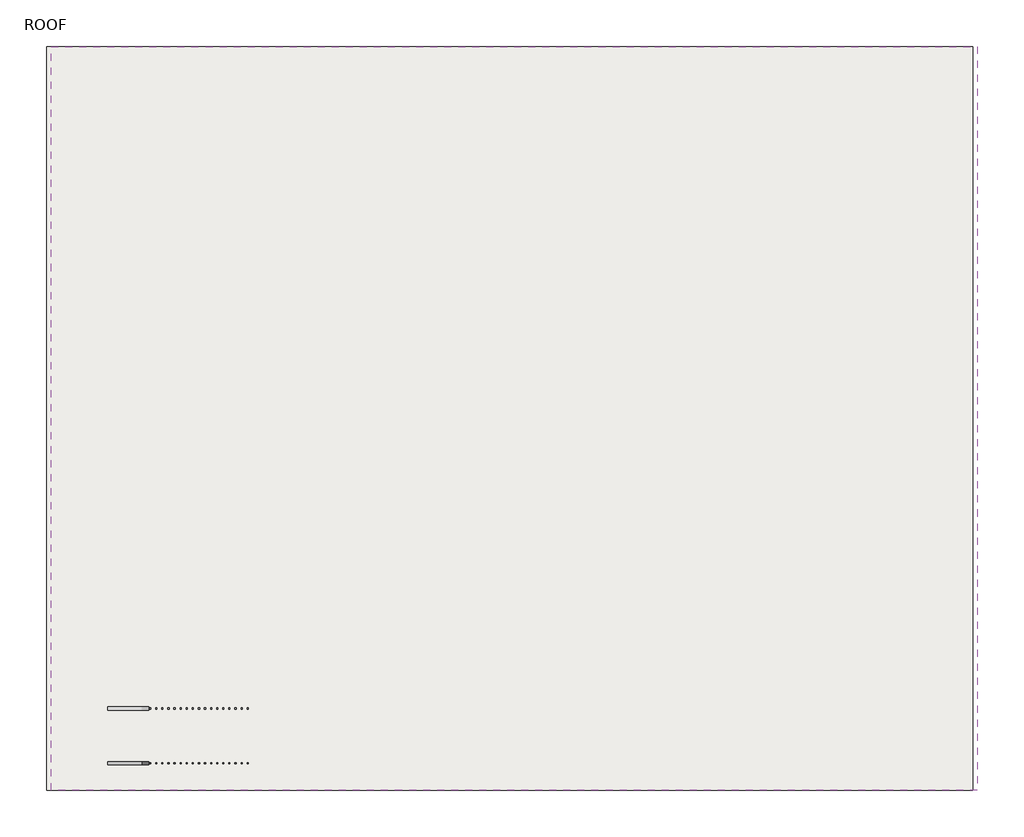
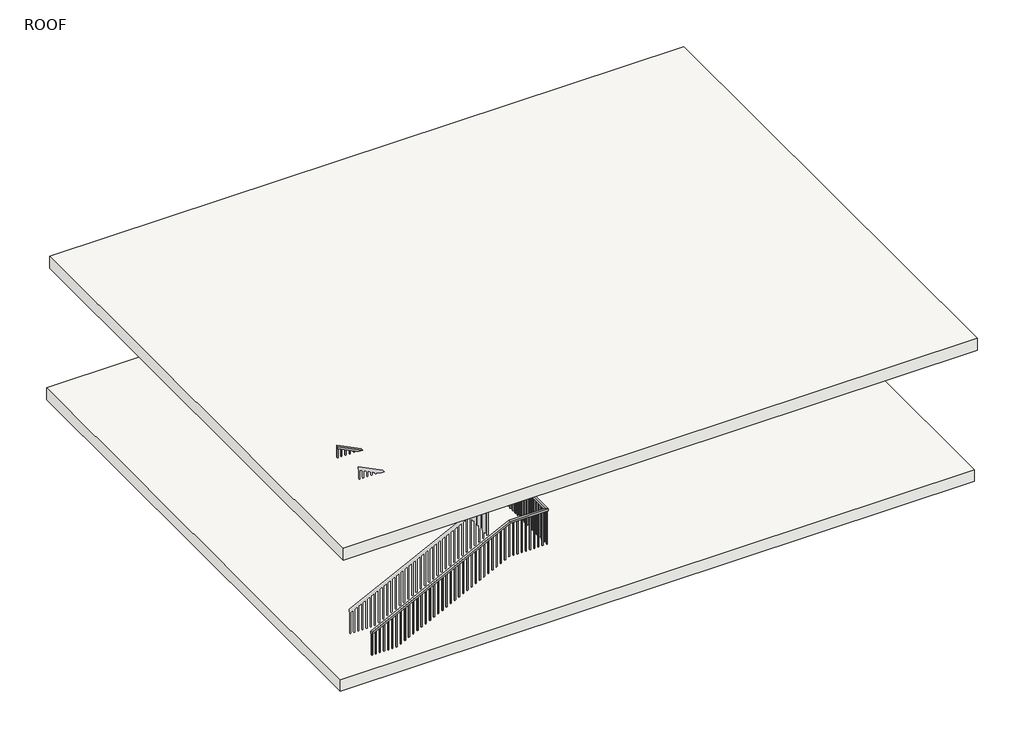
# One storey, part 1 of 2: 2 slabs, 1 railing.
"""IFC4 building model written with IfcOpenShell, lengths in millimetres."""

from ifc_helpers import new_model, si_unit, frame, origin, place, context, project, spatial, polyline, outline, extrude, faceted_brep, element, save

model = new_model("IFC4")

# Units and contexts
model_context = context("Model", 3, world=origin())
ifc_project = project(units=[si_unit("LENGTHUNIT", "METRE", prefix="MILLI")], contexts=[model_context])

# Site, building, storey
site = spatial("IfcSite", under=ifc_project)
building = spatial("IfcBuilding", under=site)
storey = spatial("IfcBuildingStorey", under=building, Name="ROOF", Elevation=12192.0)

# Railing
placement = place(None, origin())
element("IfcRailing", 1, ObjectType="Handrail - Rectangular", at=placement, inside=storey, context=model_context, shape_type="SolidModel", body=[
    faceted_brep([(-8362.2800418, -5370.1090076, 13106.4), (-8362.2800418, -5370.1090076, 13049.6038734), (-8362.2800418, -5420.9090076, 13049.6038734), (-8362.2800418, -5420.9090076, 13106.4), (-5009.4800418, -5370.1090076, 14782.8), (-4997.4877885, -5370.1090076, 14732.0), (-4997.4877885, -5420.9090076, 14732.0), (-5009.4800418, -5420.9090076, 14782.8), (-4120.4800418, -5370.1090076, 14782.8), (-4120.4800418, -5370.1090076, 14732.0), (-4069.6800418, -5420.9090076, 14732.0), (-4069.6800418, -5420.9090076, 14782.8), (-4120.4800418, -2917.1346494, 14782.8), (-4120.4800418, -2917.1346494, 14732.0), (-4069.6800418, -2866.3346494, 14732.0), (-4069.6800418, -2866.3346494, 14782.8), (-5009.4800418, -2917.1346494, 14782.8), (-5021.472295, -2917.1346494, 14732.0), (-5021.472295, -2866.3346494, 14732.0), (-5009.4800418, -2866.3346494, 14782.8), (-7752.6800418, -2917.1346494, 16154.4), (-7752.6800418, -2866.3346494, 16154.4), (-7752.6800418, -2866.3346494, 16097.6038734), (-7752.6800418, -2917.1346494, 16097.6038734)], [[[0, 1, 2, 3]], [[1, 0, 4, 5]], [[2, 1, 5, 6]], [[3, 2, 6, 7]], [[0, 3, 7, 4]], [[5, 4, 8, 9]], [[6, 5, 9, 10]], [[7, 6, 10, 11]], [[4, 7, 11, 8]], [[9, 8, 12, 13]], [[10, 9, 13, 14]], [[11, 10, 14, 15]], [[8, 11, 15, 12]], [[13, 12, 16, 17]], [[14, 13, 17, 18]], [[15, 14, 18, 19]], [[12, 15, 19, 16]], [[20, 21, 22, 23]], [[17, 16, 20, 23]], [[18, 17, 23, 22]], [[19, 18, 22, 21]], [[16, 19, 21, 20]]]),
    extrude(outline(polyline([(16051.5663734, -7660.6050418), (15193.9625, -7660.6050418), (15184.4375, -7641.5550418), (16042.0413734, -7641.5550418), (16051.5663734, -7660.6050418)])), frame((0.0, -2901.2596494, 0.0), z_axis=(0.0, 1.0, 0.0), x_axis=(0.0, 0.0, 1.0)), (0.0, 0.0, 1.0), 19.05),
    extrude(outline(polyline([(16000.7663734, -7559.0050418), (15143.1625, -7559.0050418), (15133.6375, -7539.9550418), (15991.2413734, -7539.9550418), (16000.7663734, -7559.0050418)])), frame((0.0, -2901.2596494, 0.0), z_axis=(0.0, 1.0, 0.0), x_axis=(0.0, 0.0, 1.0)), (0.0, 0.0, 1.0), 19.05),
    extrude(outline(polyline([(15949.9663734, -7457.4050418), (15092.3625, -7457.4050418), (15082.8375, -7438.3550418), (15940.4413734, -7438.3550418), (15949.9663734, -7457.4050418)])), frame((0.0, -2901.2596494, 0.0), z_axis=(0.0, 1.0, 0.0), x_axis=(0.0, 0.0, 1.0)), (0.0, 0.0, 1.0), 19.05),
    extrude(outline(polyline([(15899.1663734, -7355.8050418), (15041.5625, -7355.8050418), (15032.0375, -7336.7550418), (15889.6413734, -7336.7550418), (15899.1663734, -7355.8050418)])), frame((0.0, -2901.2596494, 0.0), z_axis=(0.0, 1.0, 0.0), x_axis=(0.0, 0.0, 1.0)), (0.0, 0.0, 1.0), 19.05),
    extrude(outline(polyline([(15848.3663734, -7254.2050418), (14990.7625, -7254.2050418), (14981.2375, -7235.1550418), (15838.8413734, -7235.1550418), (15848.3663734, -7254.2050418)])), frame((0.0, -2901.2596494, 0.0), z_axis=(0.0, 1.0, 0.0), x_axis=(0.0, 0.0, 1.0)), (0.0, 0.0, 1.0), 19.05),
    extrude(outline(polyline([(15797.5663734, -7152.6050418), (14939.9625, -7152.6050418), (14930.4375, -7133.5550418), (15788.0413734, -7133.5550418), (15797.5663734, -7152.6050418)])), frame((0.0, -2901.2596494, 0.0), z_axis=(0.0, 1.0, 0.0), x_axis=(0.0, 0.0, 1.0)), (0.0, 0.0, 1.0), 19.05),
    extrude(outline(polyline([(15746.7663734, -7051.0050418), (14889.1625, -7051.0050418), (14879.6375, -7031.9550418), (15737.2413734, -7031.9550418), (15746.7663734, -7051.0050418)])), frame((0.0, -2901.2596494, 0.0), z_axis=(0.0, 1.0, 0.0), x_axis=(0.0, 0.0, 1.0)), (0.0, 0.0, 1.0), 19.05),
    extrude(outline(polyline([(15695.9663734, -6949.4050418), (14838.3625, -6949.4050418), (14828.8375, -6930.3550418), (15686.4413734, -6930.3550418), (15695.9663734, -6949.4050418)])), frame((0.0, -2901.2596494, 0.0), z_axis=(0.0, 1.0, 0.0), x_axis=(0.0, 0.0, 1.0)), (0.0, 0.0, 1.0), 19.05),
    extrude(outline(polyline([(15645.1663734, -6847.8050418), (14787.5625, -6847.8050418), (14778.0375, -6828.7550418), (15635.6413734, -6828.7550418), (15645.1663734, -6847.8050418)])), frame((0.0, -2901.2596494, 0.0), z_axis=(0.0, 1.0, 0.0), x_axis=(0.0, 0.0, 1.0)), (0.0, 0.0, 1.0), 19.05),
    extrude(outline(polyline([(15594.3663734, -6746.2050418), (14736.7625, -6746.2050418), (14727.2375, -6727.1550418), (15584.8413734, -6727.1550418), (15594.3663734, -6746.2050418)])), frame((0.0, -2901.2596494, 0.0), z_axis=(0.0, 1.0, 0.0), x_axis=(0.0, 0.0, 1.0)), (0.0, 0.0, 1.0), 19.05),
    extrude(outline(polyline([(15543.5663734, -6644.6050418), (14685.9625, -6644.6050418), (14676.4375, -6625.5550418), (15534.0413734, -6625.5550418), (15543.5663734, -6644.6050418)])), frame((0.0, -2901.2596494, 0.0), z_axis=(0.0, 1.0, 0.0), x_axis=(0.0, 0.0, 1.0)), (0.0, 0.0, 1.0), 19.05),
    extrude(outline(polyline([(15492.7663734, -6543.0050418), (14635.1625, -6543.0050418), (14625.6375, -6523.9550418), (15483.2413734, -6523.9550418), (15492.7663734, -6543.0050418)])), frame((0.0, -2901.2596494, 0.0), z_axis=(0.0, 1.0, 0.0), x_axis=(0.0, 0.0, 1.0)), (0.0, 0.0, 1.0), 19.05),
    extrude(outline(polyline([(15441.9663734, -6441.4050418), (14584.3625, -6441.4050418), (14574.8375, -6422.3550418), (15432.4413734, -6422.3550418), (15441.9663734, -6441.4050418)])), frame((0.0, -2901.2596494, 0.0), z_axis=(0.0, 1.0, 0.0), x_axis=(0.0, 0.0, 1.0)), (0.0, 0.0, 1.0), 19.05),
    extrude(outline(polyline([(15391.1663734, -6339.8050418), (14533.5625, -6339.8050418), (14524.0375, -6320.7550418), (15381.6413734, -6320.7550418), (15391.1663734, -6339.8050418)])), frame((0.0, -2901.2596494, 0.0), z_axis=(0.0, 1.0, 0.0), x_axis=(0.0, 0.0, 1.0)), (0.0, 0.0, 1.0), 19.05),
    extrude(outline(polyline([(15340.3663734, -6238.2050418), (14482.7625, -6238.2050418), (14473.2375, -6219.1550418), (15330.8413734, -6219.1550418), (15340.3663734, -6238.2050418)])), frame((0.0, -2901.2596494, 0.0), z_axis=(0.0, 1.0, 0.0), x_axis=(0.0, 0.0, 1.0)), (0.0, 0.0, 1.0), 19.05),
    extrude(outline(polyline([(15289.5663734, -6136.6050418), (14431.9625, -6136.6050418), (14422.4375, -6117.5550418), (15280.0413734, -6117.5550418), (15289.5663734, -6136.6050418)])), frame((0.0, -2901.2596494, 0.0), z_axis=(0.0, 1.0, 0.0), x_axis=(0.0, 0.0, 1.0)), (0.0, 0.0, 1.0), 19.05),
    extrude(outline(polyline([(15238.7663734, -6035.0050418), (14381.1625, -6035.0050418), (14371.6375, -6015.9550418), (15229.2413734, -6015.9550418), (15238.7663734, -6035.0050418)])), frame((0.0, -2901.2596494, 0.0), z_axis=(0.0, 1.0, 0.0), x_axis=(0.0, 0.0, 1.0)), (0.0, 0.0, 1.0), 19.05),
    extrude(outline(polyline([(15187.9663734, -5933.4050418), (14330.3625, -5933.4050418), (14320.8375, -5914.3550418), (15178.4413734, -5914.3550418), (15187.9663734, -5933.4050418)])), frame((0.0, -2901.2596494, 0.0), z_axis=(0.0, 1.0, 0.0), x_axis=(0.0, 0.0, 1.0)), (0.0, 0.0, 1.0), 19.05),
    extrude(outline(polyline([(15137.1663734, -5831.8050418), (14279.5625, -5831.8050418), (14270.0375, -5812.7550418), (15127.6413734, -5812.7550418), (15137.1663734, -5831.8050418)])), frame((0.0, -2901.2596494, 0.0), z_axis=(0.0, 1.0, 0.0), x_axis=(0.0, 0.0, 1.0)), (0.0, 0.0, 1.0), 19.05),
    extrude(outline(polyline([(15086.3663734, -5730.2050418), (14228.7625, -5730.2050418), (14219.2375, -5711.1550418), (15076.8413734, -5711.1550418), (15086.3663734, -5730.2050418)])), frame((0.0, -2901.2596494, 0.0), z_axis=(0.0, 1.0, 0.0), x_axis=(0.0, 0.0, 1.0)), (0.0, 0.0, 1.0), 19.05),
    extrude(outline(polyline([(15035.5663734, -5628.6050418), (14177.9625, -5628.6050418), (14168.4375, -5609.5550418), (15026.0413734, -5609.5550418), (15035.5663734, -5628.6050418)])), frame((0.0, -2901.2596494, 0.0), z_axis=(0.0, 1.0, 0.0), x_axis=(0.0, 0.0, 1.0)), (0.0, 0.0, 1.0), 19.05),
    extrude(outline(polyline([(14984.7663734, -5527.0050418), (14127.1625, -5527.0050418), (14117.6375, -5507.9550418), (14975.2413734, -5507.9550418), (14984.7663734, -5527.0050418)])), frame((0.0, -2901.2596494, 0.0), z_axis=(0.0, 1.0, 0.0), x_axis=(0.0, 0.0, 1.0)), (0.0, 0.0, 1.0), 19.05),
    extrude(outline(polyline([(14933.9663734, -5425.4050418), (14076.3625, -5425.4050418), (14066.8375, -5406.3550418), (14924.4413734, -5406.3550418), (14933.9663734, -5425.4050418)])), frame((0.0, -2901.2596494, 0.0), z_axis=(0.0, 1.0, 0.0), x_axis=(0.0, 0.0, 1.0)), (0.0, 0.0, 1.0), 19.05),
    extrude(outline(polyline([(14883.1663734, -5323.8050418), (14025.5625, -5323.8050418), (14016.0375, -5304.7550418), (14873.6413734, -5304.7550418), (14883.1663734, -5323.8050418)])), frame((0.0, -2901.2596494, 0.0), z_axis=(0.0, 1.0, 0.0), x_axis=(0.0, 0.0, 1.0)), (0.0, 0.0, 1.0), 19.05),
    extrude(outline(polyline([(14832.3663734, -5222.2050418), (13974.7625, -5222.2050418), (13965.2375, -5203.1550418), (14822.8413734, -5203.1550418), (14832.3663734, -5222.2050418)])), frame((0.0, -2901.2596494, 0.0), z_axis=(0.0, 1.0, 0.0), x_axis=(0.0, 0.0, 1.0)), (0.0, 0.0, 1.0), 19.05),
    extrude(outline(polyline([(14781.5663734, -5120.6050418), (13923.9625, -5120.6050418), (13914.4375, -5101.5550418), (14772.0413734, -5101.5550418), (14781.5663734, -5120.6050418)])), frame((0.0, -2901.2596494, 0.0), z_axis=(0.0, 1.0, 0.0), x_axis=(0.0, 0.0, 1.0)), (0.0, 0.0, 1.0), 19.05),
    extrude(outline(polyline([(-4898.3550418, -2901.2596494), (-4917.4050418, -2901.2596494), (-4917.4050418, -2882.2096494), (-4898.3550418, -2882.2096494), (-4898.3550418, -2901.2596494)])), frame((0.0, 0.0, 13868.4), z_axis=(0.0, 0.0, 1.0), x_axis=(1.0, 0.0, 0.0)), (0.0, 0.0, 1.0), 863.6),
    extrude(outline(polyline([(-4796.7550418, -2901.2596494), (-4815.8050418, -2901.2596494), (-4815.8050418, -2882.2096494), (-4796.7550418, -2882.2096494), (-4796.7550418, -2901.2596494)])), frame((0.0, 0.0, 13868.4), z_axis=(0.0, 0.0, 1.0), x_axis=(1.0, 0.0, 0.0)), (0.0, 0.0, 1.0), 863.6),
    extrude(outline(polyline([(-4695.1550418, -2901.2596494), (-4714.2050418, -2901.2596494), (-4714.2050418, -2882.2096494), (-4695.1550418, -2882.2096494), (-4695.1550418, -2901.2596494)])), frame((0.0, 0.0, 13868.4), z_axis=(0.0, 0.0, 1.0), x_axis=(1.0, 0.0, 0.0)), (0.0, 0.0, 1.0), 863.6),
    extrude(outline(polyline([(-4593.5550418, -2901.2596494), (-4612.6050418, -2901.2596494), (-4612.6050418, -2882.2096494), (-4593.5550418, -2882.2096494), (-4593.5550418, -2901.2596494)])), frame((0.0, 0.0, 13868.4), z_axis=(0.0, 0.0, 1.0), x_axis=(1.0, 0.0, 0.0)), (0.0, 0.0, 1.0), 863.6),
    extrude(outline(polyline([(-4491.9550418, -2901.2596494), (-4511.0050418, -2901.2596494), (-4511.0050418, -2882.2096494), (-4491.9550418, -2882.2096494), (-4491.9550418, -2901.2596494)])), frame((0.0, 0.0, 13868.4), z_axis=(0.0, 0.0, 1.0), x_axis=(1.0, 0.0, 0.0)), (0.0, 0.0, 1.0), 863.6),
    extrude(outline(polyline([(-4390.3550418, -2901.2596494), (-4409.4050418, -2901.2596494), (-4409.4050418, -2882.2096494), (-4390.3550418, -2882.2096494), (-4390.3550418, -2901.2596494)])), frame((0.0, 0.0, 13868.4), z_axis=(0.0, 0.0, 1.0), x_axis=(1.0, 0.0, 0.0)), (0.0, 0.0, 1.0), 863.6),
    extrude(outline(polyline([(-4288.7550418, -2901.2596494), (-4307.8050418, -2901.2596494), (-4307.8050418, -2882.2096494), (-4288.7550418, -2882.2096494), (-4288.7550418, -2901.2596494)])), frame((0.0, 0.0, 13868.4), z_axis=(0.0, 0.0, 1.0), x_axis=(1.0, 0.0, 0.0)), (0.0, 0.0, 1.0), 863.6),
    extrude(outline(polyline([(-4187.1550418, -2901.2596494), (-4206.2050418, -2901.2596494), (-4206.2050418, -2882.2096494), (-4187.1550418, -2882.2096494), (-4187.1550418, -2901.2596494)])), frame((0.0, 0.0, 13868.4), z_axis=(0.0, 0.0, 1.0), x_axis=(1.0, 0.0, 0.0)), (0.0, 0.0, 1.0), 863.6),
    extrude(outline(polyline([(-4104.6050418, -2966.6340076), (-4104.6050418, -2947.5840076), (-4085.5550418, -2947.5840076), (-4085.5550418, -2966.6340076), (-4104.6050418, -2966.6340076)])), frame((0.0, 0.0, 13868.4), z_axis=(0.0, 0.0, 1.0), x_axis=(1.0, 0.0, 0.0)), (0.0, 0.0, 1.0), 863.6),
    extrude(outline(polyline([(-4104.6050418, -3068.2340076), (-4104.6050418, -3049.1840076), (-4085.5550418, -3049.1840076), (-4085.5550418, -3068.2340076), (-4104.6050418, -3068.2340076)])), frame((0.0, 0.0, 13868.4), z_axis=(0.0, 0.0, 1.0), x_axis=(1.0, 0.0, 0.0)), (0.0, 0.0, 1.0), 863.6),
    extrude(outline(polyline([(-4104.6050418, -3169.8340076), (-4104.6050418, -3150.7840076), (-4085.5550418, -3150.7840076), (-4085.5550418, -3169.8340076), (-4104.6050418, -3169.8340076)])), frame((0.0, 0.0, 13868.4), z_axis=(0.0, 0.0, 1.0), x_axis=(1.0, 0.0, 0.0)), (0.0, 0.0, 1.0), 863.6),
    extrude(outline(polyline([(-4104.6050418, -3271.4340076), (-4104.6050418, -3252.3840076), (-4085.5550418, -3252.3840076), (-4085.5550418, -3271.4340076), (-4104.6050418, -3271.4340076)])), frame((0.0, 0.0, 13868.4), z_axis=(0.0, 0.0, 1.0), x_axis=(1.0, 0.0, 0.0)), (0.0, 0.0, 1.0), 863.6),
    extrude(outline(polyline([(-4104.6050418, -3373.0340076), (-4104.6050418, -3353.9840076), (-4085.5550418, -3353.9840076), (-4085.5550418, -3373.0340076), (-4104.6050418, -3373.0340076)])), frame((0.0, 0.0, 13868.4), z_axis=(0.0, 0.0, 1.0), x_axis=(1.0, 0.0, 0.0)), (0.0, 0.0, 1.0), 863.6),
    extrude(outline(polyline([(-4104.6050418, -3474.6340076), (-4104.6050418, -3455.5840076), (-4085.5550418, -3455.5840076), (-4085.5550418, -3474.6340076), (-4104.6050418, -3474.6340076)])), frame((0.0, 0.0, 13868.4), z_axis=(0.0, 0.0, 1.0), x_axis=(1.0, 0.0, 0.0)), (0.0, 0.0, 1.0), 863.6),
    extrude(outline(polyline([(-4104.6050418, -3576.2340076), (-4104.6050418, -3557.1840076), (-4085.5550418, -3557.1840076), (-4085.5550418, -3576.2340076), (-4104.6050418, -3576.2340076)])), frame((0.0, 0.0, 13868.4), z_axis=(0.0, 0.0, 1.0), x_axis=(1.0, 0.0, 0.0)), (0.0, 0.0, 1.0), 863.6),
    extrude(outline(polyline([(-4104.6050418, -3677.8340076), (-4104.6050418, -3658.7840076), (-4085.5550418, -3658.7840076), (-4085.5550418, -3677.8340076), (-4104.6050418, -3677.8340076)])), frame((0.0, 0.0, 13868.4), z_axis=(0.0, 0.0, 1.0), x_axis=(1.0, 0.0, 0.0)), (0.0, 0.0, 1.0), 863.6),
    extrude(outline(polyline([(-4104.6050418, -3779.4340076), (-4104.6050418, -3760.3840076), (-4085.5550418, -3760.3840076), (-4085.5550418, -3779.4340076), (-4104.6050418, -3779.4340076)])), frame((0.0, 0.0, 13868.4), z_axis=(0.0, 0.0, 1.0), x_axis=(1.0, 0.0, 0.0)), (0.0, 0.0, 1.0), 863.6),
    extrude(outline(polyline([(-4104.6050418, -3881.0340076), (-4104.6050418, -3861.9840076), (-4085.5550418, -3861.9840076), (-4085.5550418, -3881.0340076), (-4104.6050418, -3881.0340076)])), frame((0.0, 0.0, 13868.4), z_axis=(0.0, 0.0, 1.0), x_axis=(1.0, 0.0, 0.0)), (0.0, 0.0, 1.0), 863.6),
    extrude(outline(polyline([(-4104.6050418, -3982.6340076), (-4104.6050418, -3963.5840076), (-4085.5550418, -3963.5840076), (-4085.5550418, -3982.6340076), (-4104.6050418, -3982.6340076)])), frame((0.0, 0.0, 13868.4), z_axis=(0.0, 0.0, 1.0), x_axis=(1.0, 0.0, 0.0)), (0.0, 0.0, 1.0), 863.6),
    extrude(outline(polyline([(-4104.6050418, -4084.2340076), (-4104.6050418, -4065.1840076), (-4085.5550418, -4065.1840076), (-4085.5550418, -4084.2340076), (-4104.6050418, -4084.2340076)])), frame((0.0, 0.0, 13868.4), z_axis=(0.0, 0.0, 1.0), x_axis=(1.0, 0.0, 0.0)), (0.0, 0.0, 1.0), 863.6),
    extrude(outline(polyline([(-4104.6050418, -4185.8340076), (-4104.6050418, -4166.7840076), (-4085.5550418, -4166.7840076), (-4085.5550418, -4185.8340076), (-4104.6050418, -4185.8340076)])), frame((0.0, 0.0, 13868.4), z_axis=(0.0, 0.0, 1.0), x_axis=(1.0, 0.0, 0.0)), (0.0, 0.0, 1.0), 863.6),
    extrude(outline(polyline([(-4104.6050418, -4287.4340076), (-4104.6050418, -4268.3840076), (-4085.5550418, -4268.3840076), (-4085.5550418, -4287.4340076), (-4104.6050418, -4287.4340076)])), frame((0.0, 0.0, 13868.4), z_axis=(0.0, 0.0, 1.0), x_axis=(1.0, 0.0, 0.0)), (0.0, 0.0, 1.0), 863.6),
    extrude(outline(polyline([(-4104.6050418, -4389.0340076), (-4104.6050418, -4369.9840076), (-4085.5550418, -4369.9840076), (-4085.5550418, -4389.0340076), (-4104.6050418, -4389.0340076)])), frame((0.0, 0.0, 13868.4), z_axis=(0.0, 0.0, 1.0), x_axis=(1.0, 0.0, 0.0)), (0.0, 0.0, 1.0), 863.6),
    extrude(outline(polyline([(-4104.6050418, -4490.6340076), (-4104.6050418, -4471.5840076), (-4085.5550418, -4471.5840076), (-4085.5550418, -4490.6340076), (-4104.6050418, -4490.6340076)])), frame((0.0, 0.0, 13868.4), z_axis=(0.0, 0.0, 1.0), x_axis=(1.0, 0.0, 0.0)), (0.0, 0.0, 1.0), 863.6),
    extrude(outline(polyline([(-4104.6050418, -4592.2340076), (-4104.6050418, -4573.1840076), (-4085.5550418, -4573.1840076), (-4085.5550418, -4592.2340076), (-4104.6050418, -4592.2340076)])), frame((0.0, 0.0, 13868.4), z_axis=(0.0, 0.0, 1.0), x_axis=(1.0, 0.0, 0.0)), (0.0, 0.0, 1.0), 863.6),
    extrude(outline(polyline([(-4104.6050418, -4693.8340076), (-4104.6050418, -4674.7840076), (-4085.5550418, -4674.7840076), (-4085.5550418, -4693.8340076), (-4104.6050418, -4693.8340076)])), frame((0.0, 0.0, 13868.4), z_axis=(0.0, 0.0, 1.0), x_axis=(1.0, 0.0, 0.0)), (0.0, 0.0, 1.0), 863.6),
    extrude(outline(polyline([(-4104.6050418, -4795.4340076), (-4104.6050418, -4776.3840076), (-4085.5550418, -4776.3840076), (-4085.5550418, -4795.4340076), (-4104.6050418, -4795.4340076)])), frame((0.0, 0.0, 13868.4), z_axis=(0.0, 0.0, 1.0), x_axis=(1.0, 0.0, 0.0)), (0.0, 0.0, 1.0), 863.6),
    extrude(outline(polyline([(-4104.6050418, -4897.0340076), (-4104.6050418, -4877.9840076), (-4085.5550418, -4877.9840076), (-4085.5550418, -4897.0340076), (-4104.6050418, -4897.0340076)])), frame((0.0, 0.0, 13868.4), z_axis=(0.0, 0.0, 1.0), x_axis=(1.0, 0.0, 0.0)), (0.0, 0.0, 1.0), 863.6),
    extrude(outline(polyline([(-4104.6050418, -4998.6340076), (-4104.6050418, -4979.5840076), (-4085.5550418, -4979.5840076), (-4085.5550418, -4998.6340076), (-4104.6050418, -4998.6340076)])), frame((0.0, 0.0, 13868.4), z_axis=(0.0, 0.0, 1.0), x_axis=(1.0, 0.0, 0.0)), (0.0, 0.0, 1.0), 863.6),
    extrude(outline(polyline([(-4104.6050418, -5100.2340076), (-4104.6050418, -5081.1840076), (-4085.5550418, -5081.1840076), (-4085.5550418, -5100.2340076), (-4104.6050418, -5100.2340076)])), frame((0.0, 0.0, 13868.4), z_axis=(0.0, 0.0, 1.0), x_axis=(1.0, 0.0, 0.0)), (0.0, 0.0, 1.0), 863.6),
    extrude(outline(polyline([(-4104.6050418, -5201.8340076), (-4104.6050418, -5182.7840076), (-4085.5550418, -5182.7840076), (-4085.5550418, -5201.8340076), (-4104.6050418, -5201.8340076)])), frame((0.0, 0.0, 13868.4), z_axis=(0.0, 0.0, 1.0), x_axis=(1.0, 0.0, 0.0)), (0.0, 0.0, 1.0), 863.6),
    extrude(outline(polyline([(-4104.6050418, -5303.4340076), (-4104.6050418, -5284.3840076), (-4085.5550418, -5284.3840076), (-4085.5550418, -5303.4340076), (-4104.6050418, -5303.4340076)])), frame((0.0, 0.0, 13868.4), z_axis=(0.0, 0.0, 1.0), x_axis=(1.0, 0.0, 0.0)), (0.0, 0.0, 1.0), 863.6),
    extrude(outline(polyline([(-4206.2050418, -5385.9840076), (-4187.1550418, -5385.9840076), (-4187.1550418, -5405.0340076), (-4206.2050418, -5405.0340076), (-4206.2050418, -5385.9840076)])), frame((0.0, 0.0, 13868.4), z_axis=(0.0, 0.0, 1.0), x_axis=(1.0, 0.0, 0.0)), (0.0, 0.0, 1.0), 863.6),
    extrude(outline(polyline([(-4307.8050418, -5385.9840076), (-4288.7550418, -5385.9840076), (-4288.7550418, -5405.0340076), (-4307.8050418, -5405.0340076), (-4307.8050418, -5385.9840076)])), frame((0.0, 0.0, 13868.4), z_axis=(0.0, 0.0, 1.0), x_axis=(1.0, 0.0, 0.0)), (0.0, 0.0, 1.0), 863.6),
    extrude(outline(polyline([(-4409.4050418, -5385.9840076), (-4390.3550418, -5385.9840076), (-4390.3550418, -5405.0340076), (-4409.4050418, -5405.0340076), (-4409.4050418, -5385.9840076)])), frame((0.0, 0.0, 13868.4), z_axis=(0.0, 0.0, 1.0), x_axis=(1.0, 0.0, 0.0)), (0.0, 0.0, 1.0), 863.6),
    extrude(outline(polyline([(-4511.0050418, -5385.9840076), (-4491.9550418, -5385.9840076), (-4491.9550418, -5405.0340076), (-4511.0050418, -5405.0340076), (-4511.0050418, -5385.9840076)])), frame((0.0, 0.0, 13868.4), z_axis=(0.0, 0.0, 1.0), x_axis=(1.0, 0.0, 0.0)), (0.0, 0.0, 1.0), 863.6),
    extrude(outline(polyline([(-4612.6050418, -5385.9840076), (-4593.5550418, -5385.9840076), (-4593.5550418, -5405.0340076), (-4612.6050418, -5405.0340076), (-4612.6050418, -5385.9840076)])), frame((0.0, 0.0, 13868.4), z_axis=(0.0, 0.0, 1.0), x_axis=(1.0, 0.0, 0.0)), (0.0, 0.0, 1.0), 863.6),
    extrude(outline(polyline([(-4714.2050418, -5385.9840076), (-4695.1550418, -5385.9840076), (-4695.1550418, -5405.0340076), (-4714.2050418, -5405.0340076), (-4714.2050418, -5385.9840076)])), frame((0.0, 0.0, 13868.4), z_axis=(0.0, 0.0, 1.0), x_axis=(1.0, 0.0, 0.0)), (0.0, 0.0, 1.0), 863.6),
    extrude(outline(polyline([(-4815.8050418, -5385.9840076), (-4796.7550418, -5385.9840076), (-4796.7550418, -5405.0340076), (-4815.8050418, -5405.0340076), (-4815.8050418, -5385.9840076)])), frame((0.0, 0.0, 13868.4), z_axis=(0.0, 0.0, 1.0), x_axis=(1.0, 0.0, 0.0)), (0.0, 0.0, 1.0), 863.6),
    extrude(outline(polyline([(-4917.4050418, -5385.9840076), (-4898.3550418, -5385.9840076), (-4898.3550418, -5405.0340076), (-4917.4050418, -5405.0340076), (-4917.4050418, -5385.9840076)])), frame((0.0, 0.0, 13868.4), z_axis=(0.0, 0.0, 1.0), x_axis=(1.0, 0.0, 0.0)), (0.0, 0.0, 1.0), 863.6),
    extrude(outline(polyline([(14670.4413734, -5120.6050418), (13812.8375, -5120.6050418), (13822.3625, -5101.5550418), (14679.9663734, -5101.5550418), (14670.4413734, -5120.6050418)])), frame((0.0, -5405.0340076, 0.0), z_axis=(0.0, 1.0, 0.0), x_axis=(0.0, 0.0, 1.0)), (0.0, 0.0, 1.0), 19.05),
    extrude(outline(polyline([(14619.6413734, -5222.2050418), (13762.0375, -5222.2050418), (13771.5625, -5203.1550418), (14629.1663734, -5203.1550418), (14619.6413734, -5222.2050418)])), frame((0.0, -5405.0340076, 0.0), z_axis=(0.0, 1.0, 0.0), x_axis=(0.0, 0.0, 1.0)), (0.0, 0.0, 1.0), 19.05),
    extrude(outline(polyline([(14568.8413734, -5323.8050418), (13711.2375, -5323.8050418), (13720.7625, -5304.7550418), (14578.3663734, -5304.7550418), (14568.8413734, -5323.8050418)])), frame((0.0, -5405.0340076, 0.0), z_axis=(0.0, 1.0, 0.0), x_axis=(0.0, 0.0, 1.0)), (0.0, 0.0, 1.0), 19.05),
    extrude(outline(polyline([(14518.0413734, -5425.4050418), (13660.4375, -5425.4050418), (13669.9625, -5406.3550418), (14527.5663734, -5406.3550418), (14518.0413734, -5425.4050418)])), frame((0.0, -5405.0340076, 0.0), z_axis=(0.0, 1.0, 0.0), x_axis=(0.0, 0.0, 1.0)), (0.0, 0.0, 1.0), 19.05),
    extrude(outline(polyline([(14467.2413734, -5527.0050418), (13609.6375, -5527.0050418), (13619.1625, -5507.9550418), (14476.7663734, -5507.9550418), (14467.2413734, -5527.0050418)])), frame((0.0, -5405.0340076, 0.0), z_axis=(0.0, 1.0, 0.0), x_axis=(0.0, 0.0, 1.0)), (0.0, 0.0, 1.0), 19.05),
    extrude(outline(polyline([(14416.4413734, -5628.6050418), (13558.8375, -5628.6050418), (13568.3625, -5609.5550418), (14425.9663734, -5609.5550418), (14416.4413734, -5628.6050418)])), frame((0.0, -5405.0340076, 0.0), z_axis=(0.0, 1.0, 0.0), x_axis=(0.0, 0.0, 1.0)), (0.0, 0.0, 1.0), 19.05),
    extrude(outline(polyline([(14365.6413734, -5730.2050418), (13508.0375, -5730.2050418), (13517.5625, -5711.1550418), (14375.1663734, -5711.1550418), (14365.6413734, -5730.2050418)])), frame((0.0, -5405.0340076, 0.0), z_axis=(0.0, 1.0, 0.0), x_axis=(0.0, 0.0, 1.0)), (0.0, 0.0, 1.0), 19.05),
    extrude(outline(polyline([(14314.8413734, -5831.8050418), (13457.2375, -5831.8050418), (13466.7625, -5812.7550418), (14324.3663734, -5812.7550418), (14314.8413734, -5831.8050418)])), frame((0.0, -5405.0340076, 0.0), z_axis=(0.0, 1.0, 0.0), x_axis=(0.0, 0.0, 1.0)), (0.0, 0.0, 1.0), 19.05),
    extrude(outline(polyline([(14264.0413734, -5933.4050418), (13406.4375, -5933.4050418), (13415.9625, -5914.3550418), (14273.5663734, -5914.3550418), (14264.0413734, -5933.4050418)])), frame((0.0, -5405.0340076, 0.0), z_axis=(0.0, 1.0, 0.0), x_axis=(0.0, 0.0, 1.0)), (0.0, 0.0, 1.0), 19.05),
    extrude(outline(polyline([(14213.2413734, -6035.0050418), (13355.6375, -6035.0050418), (13365.1625, -6015.9550418), (14222.7663734, -6015.9550418), (14213.2413734, -6035.0050418)])), frame((0.0, -5405.0340076, 0.0), z_axis=(0.0, 1.0, 0.0), x_axis=(0.0, 0.0, 1.0)), (0.0, 0.0, 1.0), 19.05),
    extrude(outline(polyline([(14162.4413734, -6136.6050418), (13304.8375, -6136.6050418), (13314.3625, -6117.5550418), (14171.9663734, -6117.5550418), (14162.4413734, -6136.6050418)])), frame((0.0, -5405.0340076, 0.0), z_axis=(0.0, 1.0, 0.0), x_axis=(0.0, 0.0, 1.0)), (0.0, 0.0, 1.0), 19.05),
    extrude(outline(polyline([(14111.6413734, -6238.2050418), (13254.0375, -6238.2050418), (13263.5625, -6219.1550418), (14121.1663734, -6219.1550418), (14111.6413734, -6238.2050418)])), frame((0.0, -5405.0340076, 0.0), z_axis=(0.0, 1.0, 0.0), x_axis=(0.0, 0.0, 1.0)), (0.0, 0.0, 1.0), 19.05),
    extrude(outline(polyline([(14060.8413734, -6339.8050418), (13203.2375, -6339.8050418), (13212.7625, -6320.7550418), (14070.3663734, -6320.7550418), (14060.8413734, -6339.8050418)])), frame((0.0, -5405.0340076, 0.0), z_axis=(0.0, 1.0, 0.0), x_axis=(0.0, 0.0, 1.0)), (0.0, 0.0, 1.0), 19.05),
    extrude(outline(polyline([(14010.0413734, -6441.4050418), (13152.4375, -6441.4050418), (13161.9625, -6422.3550418), (14019.5663734, -6422.3550418), (14010.0413734, -6441.4050418)])), frame((0.0, -5405.0340076, 0.0), z_axis=(0.0, 1.0, 0.0), x_axis=(0.0, 0.0, 1.0)), (0.0, 0.0, 1.0), 19.05),
    extrude(outline(polyline([(13959.2413734, -6543.0050418), (13101.6375, -6543.0050418), (13111.1625, -6523.9550418), (13968.7663734, -6523.9550418), (13959.2413734, -6543.0050418)])), frame((0.0, -5405.0340076, 0.0), z_axis=(0.0, 1.0, 0.0), x_axis=(0.0, 0.0, 1.0)), (0.0, 0.0, 1.0), 19.05),
    extrude(outline(polyline([(13908.4413734, -6644.6050418), (13050.8375, -6644.6050418), (13060.3625, -6625.5550418), (13917.9663734, -6625.5550418), (13908.4413734, -6644.6050418)])), frame((0.0, -5405.0340076, 0.0), z_axis=(0.0, 1.0, 0.0), x_axis=(0.0, 0.0, 1.0)), (0.0, 0.0, 1.0), 19.05),
    extrude(outline(polyline([(13857.6413734, -6746.2050418), (13000.0375, -6746.2050418), (13009.5625, -6727.1550418), (13867.1663734, -6727.1550418), (13857.6413734, -6746.2050418)])), frame((0.0, -5405.0340076, 0.0), z_axis=(0.0, 1.0, 0.0), x_axis=(0.0, 0.0, 1.0)), (0.0, 0.0, 1.0), 19.05),
    extrude(outline(polyline([(13806.8413734, -6847.8050418), (12949.2375, -6847.8050418), (12958.7625, -6828.7550418), (13816.3663734, -6828.7550418), (13806.8413734, -6847.8050418)])), frame((0.0, -5405.0340076, 0.0), z_axis=(0.0, 1.0, 0.0), x_axis=(0.0, 0.0, 1.0)), (0.0, 0.0, 1.0), 19.05),
    extrude(outline(polyline([(13756.0413734, -6949.4050418), (12898.4375, -6949.4050418), (12907.9625, -6930.3550418), (13765.5663734, -6930.3550418), (13756.0413734, -6949.4050418)])), frame((0.0, -5405.0340076, 0.0), z_axis=(0.0, 1.0, 0.0), x_axis=(0.0, 0.0, 1.0)), (0.0, 0.0, 1.0), 19.05),
    extrude(outline(polyline([(13705.2413734, -7051.0050418), (12847.6375, -7051.0050418), (12857.1625, -7031.9550418), (13714.7663734, -7031.9550418), (13705.2413734, -7051.0050418)])), frame((0.0, -5405.0340076, 0.0), z_axis=(0.0, 1.0, 0.0), x_axis=(0.0, 0.0, 1.0)), (0.0, 0.0, 1.0), 19.05),
    extrude(outline(polyline([(13654.4413734, -7152.6050418), (12796.8375, -7152.6050418), (12806.3625, -7133.5550418), (13663.9663734, -7133.5550418), (13654.4413734, -7152.6050418)])), frame((0.0, -5405.0340076, 0.0), z_axis=(0.0, 1.0, 0.0), x_axis=(0.0, 0.0, 1.0)), (0.0, 0.0, 1.0), 19.05),
    extrude(outline(polyline([(13603.6413734, -7254.2050418), (12746.0375, -7254.2050418), (12755.5625, -7235.1550418), (13613.1663734, -7235.1550418), (13603.6413734, -7254.2050418)])), frame((0.0, -5405.0340076, 0.0), z_axis=(0.0, 1.0, 0.0), x_axis=(0.0, 0.0, 1.0)), (0.0, 0.0, 1.0), 19.05),
    extrude(outline(polyline([(13552.8413734, -7355.8050418), (12695.2375, -7355.8050418), (12704.7625, -7336.7550418), (13562.3663734, -7336.7550418), (13552.8413734, -7355.8050418)])), frame((0.0, -5405.0340076, 0.0), z_axis=(0.0, 1.0, 0.0), x_axis=(0.0, 0.0, 1.0)), (0.0, 0.0, 1.0), 19.05),
    extrude(outline(polyline([(13502.0413734, -7457.4050418), (12644.4375, -7457.4050418), (12653.9625, -7438.3550418), (13511.5663734, -7438.3550418), (13502.0413734, -7457.4050418)])), frame((0.0, -5405.0340076, 0.0), z_axis=(0.0, 1.0, 0.0), x_axis=(0.0, 0.0, 1.0)), (0.0, 0.0, 1.0), 19.05),
    extrude(outline(polyline([(13451.2413734, -7559.0050418), (12593.6375, -7559.0050418), (12603.1625, -7539.9550418), (13460.7663734, -7539.9550418), (13451.2413734, -7559.0050418)])), frame((0.0, -5405.0340076, 0.0), z_axis=(0.0, 1.0, 0.0), x_axis=(0.0, 0.0, 1.0)), (0.0, 0.0, 1.0), 19.05),
    extrude(outline(polyline([(13400.4413734, -7660.6050418), (12542.8375, -7660.6050418), (12552.3625, -7641.5550418), (13409.9663734, -7641.5550418), (13400.4413734, -7660.6050418)])), frame((0.0, -5405.0340076, 0.0), z_axis=(0.0, 1.0, 0.0), x_axis=(0.0, 0.0, 1.0)), (0.0, 0.0, 1.0), 19.05),
    extrude(outline(polyline([(13349.6413734, -7762.2050418), (12492.0375, -7762.2050418), (12501.5625, -7743.1550418), (13359.1663734, -7743.1550418), (13349.6413734, -7762.2050418)])), frame((0.0, -5405.0340076, 0.0), z_axis=(0.0, 1.0, 0.0), x_axis=(0.0, 0.0, 1.0)), (0.0, 0.0, 1.0), 19.05),
    extrude(outline(polyline([(13298.8413734, -7863.8050418), (12441.2375, -7863.8050418), (12450.7625, -7844.7550418), (13308.3663734, -7844.7550418), (13298.8413734, -7863.8050418)])), frame((0.0, -5405.0340076, 0.0), z_axis=(0.0, 1.0, 0.0), x_axis=(0.0, 0.0, 1.0)), (0.0, 0.0, 1.0), 19.05),
    extrude(outline(polyline([(13248.0413734, -7965.4050418), (12390.4375, -7965.4050418), (12399.9625, -7946.3550418), (13257.5663734, -7946.3550418), (13248.0413734, -7965.4050418)])), frame((0.0, -5405.0340076, 0.0), z_axis=(0.0, 1.0, 0.0), x_axis=(0.0, 0.0, 1.0)), (0.0, 0.0, 1.0), 19.05),
    extrude(outline(polyline([(13197.2413734, -8067.0050418), (12339.6375, -8067.0050418), (12349.1625, -8047.9550418), (13206.7663734, -8047.9550418), (13197.2413734, -8067.0050418)])), frame((0.0, -5405.0340076, 0.0), z_axis=(0.0, 1.0, 0.0), x_axis=(0.0, 0.0, 1.0)), (0.0, 0.0, 1.0), 19.05),
    extrude(outline(polyline([(13146.4413734, -8168.6050418), (12288.8375, -8168.6050418), (12298.3625, -8149.5550418), (13155.9663734, -8149.5550418), (13146.4413734, -8168.6050418)])), frame((0.0, -5405.0340076, 0.0), z_axis=(0.0, 1.0, 0.0), x_axis=(0.0, 0.0, 1.0)), (0.0, 0.0, 1.0), 19.05),
    extrude(outline(polyline([(13095.6413734, -8270.2050418), (12238.0375, -8270.2050418), (12247.5625, -8251.1550418), (13105.1663734, -8251.1550418), (13095.6413734, -8270.2050418)])), frame((0.0, -5405.0340076, 0.0), z_axis=(0.0, 1.0, 0.0), x_axis=(0.0, 0.0, 1.0)), (0.0, 0.0, 1.0), 19.05),
    extrude(outline(polyline([(-4999.9550418, -2901.2596494), (-5019.0050418, -2901.2596494), (-5019.0050418, -2882.2096494), (-4999.9550418, -2882.2096494), (-4999.9550418, -2901.2596494)])), frame((0.0, 0.0, 13868.4), z_axis=(0.0, 0.0, 1.0), x_axis=(1.0, 0.0, 0.0)), (0.0, 0.0, 1.0), 863.6),
    extrude(outline(polyline([(-4104.6050418, -2901.2596494), (-4104.6050418, -2882.2096494), (-4085.5550418, -2882.2096494), (-4085.5550418, -2901.2596494), (-4104.6050418, -2901.2596494)])), frame((0.0, 0.0, 13868.4), z_axis=(0.0, 0.0, 1.0), x_axis=(1.0, 0.0, 0.0)), (0.0, 0.0, 1.0), 863.6),
    extrude(outline(polyline([(-4104.6050418, -5385.9840076), (-4085.5550418, -5385.9840076), (-4085.5550418, -5405.0340076), (-4104.6050418, -5405.0340076), (-4104.6050418, -5385.9840076)])), frame((0.0, 0.0, 13868.4), z_axis=(0.0, 0.0, 1.0), x_axis=(1.0, 0.0, 0.0)), (0.0, 0.0, 1.0), 863.6),
    extrude(outline(polyline([(14721.2413734, -5019.0050418), (13863.6375, -5019.0050418), (13873.1625, -4999.9550418), (14730.7663734, -4999.9550418), (14721.2413734, -5019.0050418)])), frame((0.0, -5405.0340076, 0.0), z_axis=(0.0, 1.0, 0.0), x_axis=(0.0, 0.0, 1.0)), (0.0, 0.0, 1.0), 19.05),
    extrude(outline(polyline([(16097.6038734, -7752.6800418), (15240.0, -7752.6800418), (15230.475, -7733.6300418), (16088.0788734, -7733.6300418), (16097.6038734, -7752.6800418)])), frame((0.0, -2901.2596494, 0.0), z_axis=(0.0, 1.0, 0.0), x_axis=(0.0, 0.0, 1.0)), (0.0, 0.0, 1.0), 19.05),
    extrude(outline(polyline([(13049.6038734, -8362.2800418), (12192.0, -8362.2800418), (12201.525, -8343.2300418), (13059.1288734, -8343.2300418), (13049.6038734, -8362.2800418)])), frame((0.0, -5405.0340076, 0.0), z_axis=(0.0, 1.0, 0.0), x_axis=(0.0, 0.0, 1.0)), (0.0, 0.0, 1.0), 19.05),
])

# Slabs
element("IfcSlab", 2, ObjectType="Generic - 12\"", at=placement, inside=storey, context=model_context, shape_type="SweptSolid", body=[
    extrude(outline(polyline([(6064.2982466, 6554.3761968), (6064.2982466, -5840.8238032), (-9378.9017534, -5840.8238032), (-9378.9017534, 6554.3761968), (6064.2982466, 6554.3761968)])), frame((0.0, 0.0, 12192.0), z_axis=(0.0, 0.0, 1.0), x_axis=(1.0, 0.0, 0.0)), (0.0, 0.0, 1.0), 304.8),
])
element("IfcSlab", 3, ObjectType="Generic - 12\"", at=placement, inside=storey, context=model_context, shape_type="SweptSolid", body=[
    extrude(outline(polyline([(6140.4982466, 6554.3761968), (6140.4982466, -5840.8238032), (-9302.7017534, -5840.8238032), (-9302.7017534, 6554.3761968), (6140.4982466, 6554.3761968)])), frame((0.0, 0.0, 15544.8), z_axis=(0.0, 0.0, 1.0), x_axis=(1.0, 0.0, 0.0)), (0.0, 0.0, 1.0), 304.8),
])

save(model, "model.ifc")

# Revit data of these elements
# Type "Handrail - Rectangular"
#   Assembly Code = "C2010400"
#   built-in parameter 1008612 = 0.0416667 (stored number, unit not read)
#   built-in parameter 1008611 = 0.0416667 (stored number, unit not read)
#   built-in parameter 1008609 = 0.333333 (stored number, unit not read)
#   built-in parameter 1008604 = 0.166667 (stored number, unit not read)
#   built-in parameter 1008603 = 0.166667 (stored number, unit not read)
#   Railing Height = 3' - 0"
#   built-in parameter 1008630 = 2
#   built-in parameter 1008610 = 2
#   built-in parameter 1008618 = Baluster - Square : 3/4"
# Type "Generic - 12\""
#   Assembly Code = "B1010"
#   Function = 0
#   Layers, outside or top first: 1' - 0" no material (function 1)
# Element 1 (IfcRailing, "Handrail - Rectangular")
#   Phase Created = New Construction
# Element 2 (IfcSlab, "Generic - 12\"")
#   Height Offset From Level = 1' - 0"
#   Phase Created = New Construction
#   Materials on its faces: "Default Floor"
# Element 3 (IfcSlab, "Generic - 12\"")
#   Height Offset From Level = 12' - 0"
#   Phase Created = New Construction
#   Materials on its faces: "Default Floor"
# Materials
#   "Default Floor": colour RGB 128 128 128, transparency 0, Cost = 0
